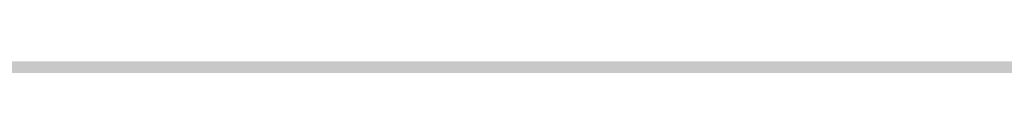
# Model space of a CAD drawing. Units: millimetres. Extents: x 0 to 2267, y 0 to 1823.
# Tile 153 of 256: x 1833.606 to 1838.83, y 1127.393 to 1127.412. Entities that reach past the tile are written whole.
import ezdxf

# ---------------------------------------------------------------- set-up
doc = ezdxf.new("R2010")
doc.units = ezdxf.units.MM
doc.header["$MEASUREMENT"] = 0
doc.layers.add('M-DIMS', color=2, linetype='Continuous', lineweight=25)
doc.layers.add('M-HATC', color=252, linetype='Continuous', lineweight=18)
doc.styles.get("Standard").update_dxf_attribs({"font": 'arial.ttf'})
doc.dimstyles.get("Standard").update_dxf_attribs({"dimtxt": 7, "dimasz": 4, "dimexe": 0.18, "dimexo": 0.0625, "dimgap": 0.09, "dimtad": 0, "dimdec": 0, "dimzin": 0, "dimdsep": 46, "dimtxsty": 'Standard', "dimcen": 0.09, "dimadec": 0, "dimazin": 0, "dimtfac": 1, "dimtdec": 0, "dimtofl": 0, "dimtmove": 0, "dimatfit": 3, "dimfxl": 1, "dimtolj": 1, "dimtzin": 0, "dimarcsym": 0})

# ---------------------------------------------------------------- blocks, each defined once
blk = doc.blocks.new('*D1')
at = {"layer": 'Defpoints', "color": 0, "transparency": 16777216}
for p in [(1593.4289, 1127.4171), (1843.4289, 1127.4171), (1843.4289, 955.6278)]:
    blk.add_point(p, dxfattribs=at)
at = {"layer": 'M-DIMS', "color": 0, "lineweight": -2, "transparency": 16777216}
for p, q in [((1593.4289, 1127.3546), (1593.4289, 955.4478)), ((1843.4289, 1127.3546), (1843.4289, 955.4478)), ((1597.4289, 955.6278), (1710.5582, 955.6278)), ((1839.4289, 955.6278), (1726.2996, 955.6278))]:
    blk.add_line(p, q, dxfattribs=at)
at = {"layer": 'M-DIMS', "color": 0, "transparency": 16777216}
for points in [[(1597.4289, 956.2944), (1597.4289, 954.9611), (1593.4289, 955.6278)], [(1839.4289, 956.2944), (1839.4289, 954.9611), (1843.4289, 955.6278)]]:
    blk.add_solid(points, dxfattribs=at)
at = {"layer": 'M-DIMS', "color": 0, "transparency": 16777216, "insert": (1718.4289, 955.6278), "char_height": 7, "attachment_point": 5}
blk.add_mtext('\\A1;250', dxfattribs=at)

msp = doc.modelspace()

# ---------------------------------------------------------------- hatches: boundary and pattern name
at = {"layer": 'M-HATC'}
h = msp.add_hatch(color=256, dxfattribs=at)
h.dxf.hatch_style = 1
h.paths.add_polyline_path([(2055.771, 1603.062), (1381.0868, 1603.062), (1381.0868, 1598.062), (2055.771, 1598.062)])
h.paths.add_polyline_path([(2055.771, 1598.062), (1381.0868, 1598.062), (1381.0868, 1593.062), (2055.771, 1593.062)])
h.paths.add_polyline_path([(2051.3074, 1536.7609), (1385.5504, 1536.7609), (1385.5504, 1526.7609), (1387.5504, 1526.7609), (1388.5366, 1525.0528), (1385.3319, 1521.2335), (1385.3319, 1521.2226), (2050.2542, 1522.7491), (2048.3212, 1525.0528), (2049.3074, 1526.7609), (2051.3074, 1526.7609)])
edge = h.paths.add_edge_path()
edge.add_arc((1847.5345, 1379.1492), 135, 222.603061, 222.890851, ccw=False)
edge.add_line((1748.1663, 1287.7656), (1683.0921, 1287.7656))
edge.add_arc((1583.7239, 1379.1492), 135, 317.109149, 317.396939, ccw=False)
edge.add_arc((1678.9686, 1290.6707), 5, 222.8909, 317.1091, ccw=False)
edge.add_arc((1774.2133, 1379.1492), 135, 222.603061, 222.890851, ccw=False)
edge.add_line((1674.8451, 1287.7656), (1609.7709, 1287.7656))
edge.add_arc((1510.4027, 1379.1492), 135, 317.109149, 317.396939, ccw=False)
edge.add_arc((1605.6474, 1290.6707), 5, 222.8909, 317.1091, ccw=False)
edge.add_arc((1700.8921, 1379.1492), 135, 222.603061, 222.890851, ccw=False)
edge.add_line((1601.5239, 1287.7656), (1536.4497, 1287.7656))
edge.add_arc((1437.0815, 1379.1492), 135, 317.109149, 317.396939, ccw=False)
edge.add_arc((1532.3262, 1290.6707), 5, 222.8909, 317.1091, ccw=False)
edge.add_arc((1627.5709, 1379.1492), 135, 222.603061, 222.890851, ccw=False)
edge.add_line((1528.2027, 1287.7656), (1505.9289, 1287.7656))
edge.add_spline(control_points=[(1505.9289, 1287.7656), (1504.2622, 1287.7656), (1504.2622, 1282.7656), (1505.9289, 1282.7656)], knot_values=[0, 0, 0, 0, 5, 5, 5, 5], degree=3, periodic=0)
edge.add_line((1505.9289, 1282.7656), (1930.9289, 1282.7656))
edge.add_spline(control_points=[(1930.9289, 1282.7656), (1932.5956, 1282.7656), (1932.5956, 1287.7656), (1930.9289, 1287.7656)], knot_values=[0, 0, 0, 0, 5, 5, 5, 5], degree=3, periodic=0)
edge.add_line((1930.9289, 1287.7656), (1903.0557, 1287.7656))
edge.add_arc((1803.6875, 1379.1492), 135, 317.109149, 317.396939, ccw=False)
edge.add_arc((1898.9322, 1290.6707), 5, 222.8909, 317.1091, ccw=False)
edge.add_arc((1994.1769, 1379.1492), 135, 222.603061, 222.890851, ccw=False)
edge.add_line((1894.8087, 1287.7656), (1829.7345, 1287.7656))
edge.add_arc((1730.3663, 1379.1492), 135, 317.109149, 317.396939, ccw=False)
edge.add_arc((1825.611, 1290.6707), 5, 222.8909, 317.1091, ccw=False)
edge.add_arc((1920.8557, 1379.1492), 135, 222.603061, 222.890851, ccw=False)
edge.add_line((1821.4875, 1287.7656), (1756.4133, 1287.7656))
edge.add_arc((1657.0451, 1379.1492), 135, 317.109149, 317.396939, ccw=False)
edge.add_arc((1752.2898, 1290.6707), 5, 222.8909, 317.1091, ccw=False)
edge = h.paths.add_edge_path()
edge.add_spline(control_points=[(1843.4289, 1227.2475), (1845.0956, 1227.2475), (1845.0956, 1232.2475), (1843.4289, 1232.2475)], knot_values=[0, 0, 0, 0, 5, 5, 5, 5], degree=3, periodic=0)
edge.add_line((1843.4289, 1232.2475), (1593.4289, 1232.2475))
edge.add_spline(control_points=[(1593.4289, 1232.2475), (1591.7622, 1232.2475), (1591.7622, 1227.2475), (1593.4289, 1227.2475)], knot_values=[0, 0, 0, 0, 5, 5, 5, 5], degree=3, periodic=0)
edge.add_line((1593.4289, 1227.2475), (1843.4289, 1227.2475))
h.paths.add_polyline_path([(1905.9289, 1127.4171), (1530.9289, 1127.4171, 0.414214), (1520.9289, 1117.4171), (1530.9289, 1117.4171), (1915.9289, 1117.4171, 0.414214)])
edge = h.paths.add_edge_path()
edge.add_arc((1397.0858, 1498.4078), 12.7299, 90.78215, 190.87871, ccw=False)
edge.add_line((1396.912, 1511.1365), (1428.0097, 1511.3488))
edge.add_line((1428.0097, 1511.3488), (1433.0097, 1511.3488))
edge.add_line((1433.0097, 1511.3488), (1434.439, 1511.3488))
edge.add_arc((1419.474, 1498.0804), 20, 41.561, 74.08211)
edge.add_line((1424.9592, 1517.3135), (1399.9351, 1517.2561))
edge.add_spline(control_points=[(1399.9307, 1517.2561), (1399.884, 1517.2131), (1399.8328, 1517.1689), (1399.7774, 1517.1236)], knot_values=[11.567499, 11.567499, 11.567499, 11.567499, 11.814249, 11.814249, 11.814249, 11.814249], degree=3, periodic=0)
edge.add_spline(control_points=[(1399.6328, 1517.0099), (1399.5831, 1516.9721), (1399.5307, 1516.9338), (1399.4759, 1516.8947)], knot_values=[11.167718, 11.167718, 11.167718, 11.167718, 11.365188, 11.365188, 11.365188, 11.365188], degree=3, periodic=0)
edge.add_spline(control_points=[(1399.3398, 1516.8001), (1399.1514, 1516.6719), (1398.9384, 1516.5377), (1398.704, 1516.3994)], knot_values=[10.376405, 10.376405, 10.376405, 10.376405, 11.00994, 11.00994, 11.00994, 11.00994], degree=3, periodic=0)
edge.add_spline(control_points=[(1398.6572, 1516.3719), (1398.5789, 1516.326), (1398.4983, 1516.2797), (1398.4155, 1516.2331)], knot_values=[10.125175, 10.125175, 10.125175, 10.125175, 10.334406, 10.334406, 10.334406, 10.334406], degree=3, periodic=0)
edge.add_spline(control_points=[(1398.2642, 1516.1487), (1398.196, 1516.1111), (1398.1263, 1516.0732), (1398.0555, 1516.0351)], knot_values=[9.832246, 9.832246, 9.832246, 9.832246, 9.999658, 9.999658, 9.999658, 9.999658], degree=3, periodic=0)
edge.add_spline(control_points=[(1397.9987, 1516.0048), (1397.7312, 1515.8621), (1397.446, 1515.7171), (1397.1466, 1515.5714)], knot_values=[9.161808, 9.161808, 9.161808, 9.161808, 9.787769, 9.787769, 9.787769, 9.787769], degree=3, periodic=0)
edge.add_spline(control_points=[(1397.1466, 1515.5714), (1396.8418, 1515.423), (1396.5222, 1515.274), (1396.1914, 1515.1262)], knot_values=[8.524455, 8.524455, 8.524455, 8.524455, 9.161808, 9.161808, 9.161808, 9.161808], degree=3, periodic=0)
edge.add_spline(control_points=[(1396.0777, 1515.0756), (1395.9854, 1515.0348), (1395.8922, 1514.994), (1395.7983, 1514.9534)], knot_values=[8.275193, 8.275193, 8.275193, 8.275193, 8.451726, 8.451726, 8.451726, 8.451726], degree=3, periodic=0)
edge.add_spline(control_points=[(1395.6018, 1514.8691), (1395.4997, 1514.8257), (1395.3968, 1514.7824), (1395.2932, 1514.7394)], knot_values=[7.962917, 7.962917, 7.962917, 7.962917, 8.152764, 8.152764, 8.152764, 8.152764], degree=3, periodic=0)
edge.add_spline(control_points=[(1395.2116, 1514.7057), (1394.8278, 1514.5475), (1394.4345, 1514.3929), (1394.0364, 1514.2442)], knot_values=[7.21254, 7.21254, 7.21254, 7.21254, 7.913148, 7.913148, 7.913148, 7.913148], degree=3, periodic=0)
edge.add_spline(control_points=[(1394.0364, 1514.2442), (1393.7076, 1514.1214), (1393.3754, 1514.0027), (1393.0427, 1513.8895)], knot_values=[6.633733, 6.633733, 6.633733, 6.633733, 7.21254, 7.21254, 7.21254, 7.21254], degree=3, periodic=0)
edge.add_spline(control_points=[(1392.8214, 1513.815), (1392.7198, 1513.7812), (1392.6181, 1513.7479), (1392.5166, 1513.7152)], knot_values=[6.328796, 6.328796, 6.328796, 6.328796, 6.505493, 6.505493, 6.505493, 6.505493], degree=3, periodic=0)
edge.add_spline(control_points=[(1392.5166, 1513.7152), (1392.3187, 1513.6515), (1392.1212, 1513.59), (1391.9244, 1513.531)], knot_values=[5.984605, 5.984605, 5.984605, 5.984605, 6.328796, 6.328796, 6.328796, 6.328796], degree=3, periodic=0)
edge.add_spline(control_points=[(1391.7915, 1513.4915), (1391.3122, 1513.3501), (1390.8384, 1513.2239), (1390.3784, 1513.1171)], knot_values=[5.066697, 5.066697, 5.066697, 5.066697, 5.907055, 5.907055, 5.907055, 5.907055], degree=3, periodic=0)
edge.add_spline(control_points=[(1390.3784, 1513.1171), (1390.1797, 1513.071), (1389.9836, 1513.0284), (1389.7907, 1512.9899)], knot_values=[4.70367, 4.70367, 4.70367, 4.70367, 5.066695, 5.066695, 5.066695, 5.066695], degree=3, periodic=0)
edge.add_spline(control_points=[(1389.422, 1512.9204), (1389.2459, 1512.8892), (1389.0729, 1512.8617), (1388.9036, 1512.8381)], knot_values=[4.130571, 4.130571, 4.130571, 4.130571, 4.469816, 4.469816, 4.469816, 4.469816], degree=3, periodic=0)
edge.add_spline(control_points=[(1388.9036, 1512.8381), (1388.591, 1512.7946), (1388.2911, 1512.7644), (1388.0071, 1512.7494)], knot_values=[3.504031, 3.504031, 3.504031, 3.504031, 4.130571, 4.130571, 4.130571, 4.130571], degree=3, periodic=0)
edge.add_spline(control_points=[(1387.9356, 1512.7459), (1387.8538, 1512.7423), (1387.7733, 1512.74), (1387.6944, 1512.739)], knot_values=[3.268866, 3.268866, 3.268866, 3.268866, 3.451164, 3.451164, 3.451164, 3.451164], degree=3, periodic=0)
edge.add_spline(control_points=[(1387.3351, 1512.7443), (1387.2076, 1512.7499), (1387.0847, 1512.7597), (1386.967, 1512.7739)], knot_values=[2.670686, 2.670686, 2.670686, 2.670686, 2.984, 2.984, 2.984, 2.984], degree=3, periodic=0)
edge.add_spline(control_points=[(1386.8327, 1512.7922), (1386.8209, 1512.7941), (1386.8092, 1512.7959), (1386.7975, 1512.7979)], knot_values=[2.516981, 2.516981, 2.516981, 2.516981, 2.549528, 2.549528, 2.549528, 2.549528], degree=3, periodic=0)
edge.add_spline(control_points=[(1386.4526, 1512.8735), (1386.4257, 1512.881), (1386.3993, 1512.889), (1386.3733, 1512.8972)], knot_values=[2.095869, 2.095869, 2.095869, 2.095869, 2.17941, 2.17941, 2.17941, 2.17941], degree=3, periodic=0)
edge.add_spline(control_points=[(1386.0691, 1513.0189), (1386.0634, 1513.0217), (1386.0577, 1513.0246), (1386.052, 1513.0275)], knot_values=[1.72453, 1.72453, 1.72453, 1.72453, 1.745933, 1.745933, 1.745933, 1.745933], degree=3, periodic=0)
edge.add_arc((1399.474, 1498.0804), 20, 131.82432, 180)
edge.add_arc((1630.3336, 1505.5484), 250.9708, 181.705176, 236.427975)
edge.add_arc((1605.3399, 1483.3044), 218.7822, 238.660829, 243.34961)
edge.add_arc((1647.0911, 1510.3592), 262.8986, 183.129836, 237.853442, ccw=False)
h.paths.add_polyline_path([(1406.5369, 1391.9644, 0.149382), (1491.5506, 1296.4418, -0.129517)], flags=17)
edge = h.paths.add_edge_path()
edge.add_arc((2037.3838, 1498.0804), 20, 0, 48.26587)
edge.add_spline(control_points=[(2050.6973, 1513.0052), (2050.6512, 1512.9847), (2050.6034, 1512.9655), (2050.5539, 1512.9477)], knot_values=[1.835652, 1.835652, 1.835652, 1.835652, 2.000781, 2.000781, 2.000781, 2.000781], degree=3, periodic=0)
edge.add_spline(control_points=[(2050.4616, 1512.9166), (2050.479, 1512.9221), (2050.4963, 1512.9277), (2050.5133, 1512.9335)], knot_values=[2.045477, 2.045477, 2.045477, 2.045477, 2.101389, 2.101389, 2.101389, 2.101389], degree=3, periodic=0)
edge.add_spline(control_points=[(2050.129, 1512.8342), (2050.1984, 1512.8473), (2050.2657, 1512.8623), (2050.3308, 1512.8792)], knot_values=[2.237629, 2.237629, 2.237629, 2.237629, 2.435841, 2.435841, 2.435841, 2.435841], degree=3, periodic=0)
edge.add_spline(control_points=[(2050.0946, 1512.8278), (2050.1061, 1512.8299), (2050.1176, 1512.832), (2050.129, 1512.8342)], knot_values=[2.435841, 2.435841, 2.435841, 2.435841, 2.468321, 2.468321, 2.468321, 2.468321], degree=3, periodic=0)
edge.add_spline(control_points=[(2049.7843, 1512.7851), (2049.8552, 1512.7922), (2049.9243, 1512.8008), (2049.9917, 1512.8109)], knot_values=[2.563852, 2.563852, 2.563852, 2.563852, 2.748541, 2.748541, 2.748541, 2.748541], degree=3, periodic=0)
edge.add_spline(control_points=[(2049.4052, 1512.7617), (2049.5364, 1512.7653), (2049.6629, 1512.773), (2049.7843, 1512.7851)], knot_values=[2.748541, 2.748541, 2.748541, 2.748541, 3.064882, 3.064882, 3.064882, 3.064882], degree=3, periodic=0)
edge.add_spline(control_points=[(2049.1698, 1512.7597), (2049.2336, 1512.7591), (2049.2965, 1512.7594), (2049.3584, 1512.7606)], knot_values=[3.102309, 3.102309, 3.102309, 3.102309, 3.2503, 3.2503, 3.2503, 3.2503], degree=3, periodic=0)
edge.add_spline(control_points=[(2048.8573, 1512.7691), (2048.9638, 1512.7638), (2049.068, 1512.7606), (2049.1698, 1512.7597)], knot_values=[3.2503, 3.2503, 3.2503, 3.2503, 3.486069, 3.486069, 3.486069, 3.486069], degree=3, periodic=0)
edge.add_spline(control_points=[(2048.6924, 1512.7789), (2048.3729, 1512.8009), (2048.0345, 1512.8411), (2047.6817, 1512.897)], knot_values=[3.606429, 3.606429, 3.606429, 3.606429, 4.2989, 4.2989, 4.2989, 4.2989], degree=3, periodic=0)
edge.add_spline(control_points=[(2047.6817, 1512.897), (2047.5458, 1512.9185), (2047.4077, 1512.9424), (2047.2678, 1512.9685)], knot_values=[4.2989, 4.2989, 4.2989, 4.2989, 4.565769, 4.565769, 4.565769, 4.565769], degree=3, periodic=0)
edge.add_spline(control_points=[(2047.2678, 1512.9685), (2047.1449, 1512.9914), (2047.0207, 1513.016), (2046.8951, 1513.0422)], knot_values=[4.565769, 4.565769, 4.565769, 4.565769, 4.799971, 4.799971, 4.799971, 4.799971], degree=3, periodic=0)
edge.add_spline(control_points=[(2046.8951, 1513.0422), (2046.5286, 1513.1188), (2046.1513, 1513.209), (2045.7676, 1513.3107)], knot_values=[4.799971, 4.799971, 4.799971, 4.799971, 5.483718, 5.483718, 5.483718, 5.483718], degree=3, periodic=0)
edge.add_spline(control_points=[(2045.7676, 1513.3107), (2045.3724, 1513.4154), (2044.9704, 1513.5322), (2044.5662, 1513.6588)], knot_values=[5.483718, 5.483718, 5.483718, 5.483718, 6.187866, 6.187866, 6.187866, 6.187866], degree=3, periodic=0)
edge.add_spline(control_points=[(2044.5662, 1513.6588), (2044.4149, 1513.7061), (2044.2633, 1513.7549), (2044.1116, 1513.8048)], knot_values=[6.187866, 6.187866, 6.187866, 6.187866, 6.451551, 6.451551, 6.451551, 6.451551], degree=3, periodic=0)
edge.add_spline(control_points=[(2044.1116, 1513.8048), (2043.9967, 1513.8427), (2043.8817, 1513.8813), (2043.7668, 1513.9205)], knot_values=[6.451551, 6.451551, 6.451551, 6.451551, 6.651434, 6.651434, 6.651434, 6.651434], degree=3, periodic=0)
edge.add_spline(control_points=[(2043.7668, 1513.9205), (2043.3716, 1514.0554), (2042.9774, 1514.1979), (2042.5886, 1514.3458)], knot_values=[6.651434, 6.651434, 6.651434, 6.651434, 7.338879, 7.338879, 7.338879, 7.338879], degree=3, periodic=0)
edge.add_spline(control_points=[(2042.5886, 1514.3458), (2042.1643, 1514.5071), (2041.7465, 1514.6749), (2041.3409, 1514.846)], knot_values=[7.338879, 7.338879, 7.338879, 7.338879, 8.089209, 8.089209, 8.089209, 8.089209], degree=3, periodic=0)
edge.add_spline(control_points=[(2041.3409, 1514.846), (2041.1028, 1514.9465), (2040.869, 1515.0481), (2040.6405, 1515.1502)], knot_values=[8.089209, 8.089209, 8.089209, 8.089209, 8.529587, 8.529587, 8.529587, 8.529587], degree=3, periodic=0)
edge.add_spline(control_points=[(2040.51, 1515.2089), (2040.0824, 1515.4022), (2039.6747, 1515.5971), (2039.295, 1515.7894)], knot_values=[8.613818, 8.613818, 8.613818, 8.613818, 9.44571, 9.44571, 9.44571, 9.44571], degree=3, periodic=0)
edge.add_spline(control_points=[(2039.295, 1515.7894), (2039.0618, 1515.9075), (2038.8391, 1516.0246), (2038.6288, 1516.1398)], knot_values=[9.44571, 9.44571, 9.44571, 9.44571, 9.956404, 9.956404, 9.956404, 9.956404], degree=3, periodic=0)
edge.add_spline(control_points=[(2038.6288, 1516.1398), (2038.5187, 1516.2001), (2038.4121, 1516.2598), (2038.309, 1516.3189)], knot_values=[9.956404, 9.956404, 9.956404, 9.956404, 10.223542, 10.223542, 10.223542, 10.223542], degree=3, periodic=0)
edge.add_spline(control_points=[(2038.309, 1516.3189), (2038.2138, 1516.3735), (2038.1216, 1516.4276), (2038.0328, 1516.481)], knot_values=[10.223542, 10.223542, 10.223542, 10.223542, 10.47051, 10.47051, 10.47051, 10.47051], degree=3, periodic=0)
edge.add_spline(control_points=[(2038.0328, 1516.481), (2037.7855, 1516.6296), (2037.5639, 1516.773), (2037.3722, 1516.909)], knot_values=[10.47051, 10.47051, 10.47051, 10.47051, 11.15767, 11.15767, 11.15767, 11.15767], degree=3, periodic=0)
edge.add_spline(control_points=[(2037.3722, 1516.909), (2037.2789, 1516.9752), (2037.1927, 1517.0396), (2037.1142, 1517.102)], knot_values=[11.15767, 11.15767, 11.15767, 11.15767, 11.49227, 11.49227, 11.49227, 11.49227], degree=3, periodic=0)
edge.add_spline(control_points=[(2036.8564, 1517.3259), (2036.9148, 1517.2692), (2036.9814, 1517.2103), (2037.0557, 1517.1492)], knot_values=[11.577341, 11.577341, 11.577341, 11.577341, 11.91035, 11.91035, 11.91035, 11.91035], degree=3, periodic=0)
edge.add_spline(control_points=[(2036.8074, 1517.3748), (2036.823, 1517.3587), (2036.8393, 1517.3424), (2036.8564, 1517.3259)], knot_values=[11.91035, 11.91035, 11.91035, 11.91035, 12.007402, 12.007402, 12.007402, 12.007402], degree=3, periodic=0)
edge.add_spline(control_points=[(2036.7017, 1517.494), (2036.7104, 1517.483), (2036.7196, 1517.4719), (2036.7291, 1517.4606)], knot_values=[12.184155, 12.184155, 12.184155, 12.184155, 12.255409, 12.255409, 12.255409, 12.255409], degree=3, periodic=0)
edge.add_spline(control_points=[(2036.6159, 1517.6205), (2036.62, 1517.613), (2036.6243, 1517.6055), (2036.6289, 1517.5979)], knot_values=[12.487913, 12.487913, 12.487913, 12.487913, 12.541035, 12.541035, 12.541035, 12.541035], degree=3, periodic=0)
edge.add_spline(control_points=[(2036.5635, 1517.786), (2036.5637, 1517.7794), (2036.5642, 1517.7726), (2036.565, 1517.7658)], knot_values=[12.911761, 12.911761, 12.911761, 12.911761, 12.968286, 12.968286, 12.968286, 12.968286], degree=3, periodic=0)
edge.add_spline(control_points=[(2036.6166, 1517.9304), (2036.6125, 1517.9259), (2036.6086, 1517.9212), (2036.6049, 1517.9165)], knot_values=[13.382527, 13.382527, 13.382527, 13.382527, 13.433791, 13.433791, 13.433791, 13.433791], degree=3, periodic=0)
edge.add_spline(control_points=[(2036.749, 1518.017), (2036.7361, 1518.0116), (2036.7239, 1518.006), (2036.7124, 1518.0002)], knot_values=[13.726299, 13.726299, 13.726299, 13.726299, 13.809928, 13.809928, 13.809928, 13.809928], degree=3, periodic=0)
edge.add_spline(control_points=[(2036.8604, 1518.0528), (2036.8386, 1518.0474), (2036.8181, 1518.0416), (2036.7988, 1518.0353)], knot_values=[13.910887, 13.910887, 13.910887, 13.910887, 14.02153, 14.02153, 14.02153, 14.02153], degree=3, periodic=0)
edge.add_line((2036.9639, 1518.0804), (2032.3838, 1518.0804))
edge.add_line((2032.3838, 1518.0804), (2027.3838, 1518.0804))
edge.add_line((2027.3838, 1518.0804), (2022.3838, 1518.0804))
edge.add_line((2022.3838, 1518.0804), (2017.3838, 1518.0804))
edge.add_arc((2017.3838, 1498.0804), 20, 90, 138.439)
edge.add_line((2002.4188, 1511.3488), (2003.8481, 1511.3488))
edge.add_line((2003.8481, 1511.3488), (2008.8481, 1511.3488))
edge.add_line((2008.8481, 1511.3488), (2039.772, 1511.1377))
edge.add_arc((2039.772, 1498.4078), 12.7299, -10.87871, 90, ccw=False)
edge.add_arc((1789.7668, 1510.3592), 262.8986, 302.146558, 356.870164, ccw=False)
edge.add_arc((1831.5179, 1483.3044), 218.7822, 296.65039, 301.339171)
edge.add_arc((1806.5242, 1505.5484), 250.9708, 303.572025, 358.294824)
h.paths.add_polyline_path([(2030.321, 1391.9644, -0.129517), (1945.3072, 1296.4418, 0.149382)], flags=17)
edge = h.paths.add_edge_path()
edge.add_spline(control_points=[(2037.2464, 1518.0821), (2037.2898, 1518.081), (2037.3355, 1518.0804), (2037.3838, 1518.0804)], knot_values=[0.000012, 0.000012, 0.000012, 0.000012, 0.144754, 0.144754, 0.144754, 0.144754], degree=3, periodic=0)
edge.add_line((2037.3357, 1518.0804), (2037.0096, 1518.0804))
edge.add_spline(control_points=[(2037.0096, 1518.0804), (2036.9822, 1518.0768), (2036.956, 1518.0727), (2036.9312, 1518.0681)], knot_values=[14.13465, 14.13465, 14.13465, 14.13465, 14.247197, 14.247197, 14.247197, 14.247197], degree=3, periodic=0)
edge.add_spline(control_points=[(2036.9312, 1518.0681), (2036.9276, 1518.0674), (2036.9241, 1518.0667), (2036.9205, 1518.0661)], knot_values=[14.118315, 14.118315, 14.118315, 14.118315, 14.13465, 14.13465, 14.13465, 14.13465], degree=3, periodic=0)
edge.add_spline(control_points=[(2036.9205, 1518.0661), (2036.9118, 1518.0644), (2036.9032, 1518.0626), (2036.8948, 1518.0608)], knot_values=[14.078086, 14.078086, 14.078086, 14.078086, 14.118315, 14.118315, 14.118315, 14.118315], degree=3, periodic=0)
edge.add_spline(control_points=[(2036.8948, 1518.0608), (2036.883, 1518.0583), (2036.8716, 1518.0556), (2036.8604, 1518.0528)], knot_values=[14.02153, 14.02153, 14.02153, 14.02153, 14.078086, 14.078086, 14.078086, 14.078086], degree=3, periodic=0)
edge.add_spline(control_points=[(2036.8604, 1518.0528), (2036.8386, 1518.0474), (2036.8181, 1518.0416), (2036.7988, 1518.0353)], knot_values=[13.910887, 13.910887, 13.910887, 13.910887, 14.02153, 14.02153, 14.02153, 14.02153], degree=3, periodic=0)
edge.add_spline(control_points=[(2036.7988, 1518.0353), (2036.7981, 1518.035), (2036.7974, 1518.0348), (2036.7967, 1518.0346)], knot_values=[13.906906, 13.906906, 13.906906, 13.906906, 13.910887, 13.910887, 13.910887, 13.910887], degree=3, periodic=0)
edge.add_spline(control_points=[(2036.7967, 1518.0346), (2036.7882, 1518.0318), (2036.7799, 1518.0289), (2036.7719, 1518.0259)], knot_values=[13.857826, 13.857826, 13.857826, 13.857826, 13.906906, 13.906906, 13.906906, 13.906906], degree=3, periodic=0)
edge.add_spline(control_points=[(2036.7719, 1518.0259), (2036.764, 1518.023), (2036.7564, 1518.02), (2036.749, 1518.017)], knot_values=[13.809928, 13.809928, 13.809928, 13.809928, 13.857826, 13.857826, 13.857826, 13.857826], degree=3, periodic=0)
edge.add_spline(control_points=[(2036.749, 1518.017), (2036.7361, 1518.0116), (2036.7239, 1518.006), (2036.7124, 1518.0002)], knot_values=[13.726299, 13.726299, 13.726299, 13.726299, 13.809928, 13.809928, 13.809928, 13.809928], degree=3, periodic=0)
edge.add_spline(control_points=[(2036.7124, 1518.0002), (2036.7121, 1518), (2036.7118, 1517.9999), (2036.7115, 1517.9997)], knot_values=[13.723993, 13.723993, 13.723993, 13.723993, 13.726299, 13.726299, 13.726299, 13.726299], degree=3, periodic=0)
edge.add_spline(control_points=[(2036.7115, 1517.9997), (2036.7063, 1517.9971), (2036.7013, 1517.9944), (2036.6965, 1517.9917)], knot_values=[13.686536, 13.686536, 13.686536, 13.686536, 13.723993, 13.723993, 13.723993, 13.723993], degree=3, periodic=0)
edge.add_spline(control_points=[(2036.6965, 1517.9917), (2036.6919, 1517.9891), (2036.6874, 1517.9865), (2036.6831, 1517.9839)], knot_values=[13.651251, 13.651251, 13.651251, 13.651251, 13.686536, 13.686536, 13.686536, 13.686536], degree=3, periodic=0)
edge.add_spline(control_points=[(2036.6831, 1517.9839), (2036.6764, 1517.9798), (2036.67, 1517.9757), (2036.6639, 1517.9714)], knot_values=[13.596804, 13.596804, 13.596804, 13.596804, 13.651251, 13.651251, 13.651251, 13.651251], degree=3, periodic=0)
edge.add_spline(control_points=[(2036.6639, 1517.9714), (2036.6636, 1517.9712), (2036.6633, 1517.9709), (2036.6629, 1517.9707)], knot_values=[13.593956, 13.593956, 13.593956, 13.593956, 13.596804, 13.596804, 13.596804, 13.596804], degree=3, periodic=0)
edge.add_spline(control_points=[(2036.6629, 1517.9707), (2036.6603, 1517.9689), (2036.6577, 1517.967), (2036.6552, 1517.9651)], knot_values=[13.570322, 13.570322, 13.570322, 13.570322, 13.593956, 13.593956, 13.593956, 13.593956], degree=3, periodic=0)
edge.add_spline(control_points=[(2036.6552, 1517.9651), (2036.6525, 1517.9631), (2036.6499, 1517.9611), (2036.6474, 1517.9591)], knot_values=[13.545477, 13.545477, 13.545477, 13.545477, 13.570322, 13.570322, 13.570322, 13.570322], degree=3, periodic=0)
edge.add_spline(control_points=[(2036.6474, 1517.9591), (2036.6472, 1517.9589), (2036.6471, 1517.9588), (2036.6469, 1517.9587)], knot_values=[13.543931, 13.543931, 13.543931, 13.543931, 13.545477, 13.545477, 13.545477, 13.545477], degree=3, periodic=0)
edge.add_spline(control_points=[(2036.6469, 1517.9587), (2036.6412, 1517.9541), (2036.6358, 1517.9494), (2036.6307, 1517.9447)], knot_values=[13.488237, 13.488237, 13.488237, 13.488237, 13.543931, 13.543931, 13.543931, 13.543931], degree=3, periodic=0)
edge.add_spline(control_points=[(2036.6307, 1517.9447), (2036.6282, 1517.9423), (2036.6257, 1517.9399), (2036.6233, 1517.9374)], knot_values=[13.460307, 13.460307, 13.460307, 13.460307, 13.488237, 13.488237, 13.488237, 13.488237], degree=3, periodic=0)
edge.add_spline(control_points=[(2036.6233, 1517.9374), (2036.6215, 1517.9356), (2036.6198, 1517.9338), (2036.6181, 1517.932)], knot_values=[13.439712, 13.439712, 13.439712, 13.439712, 13.460307, 13.460307, 13.460307, 13.460307], degree=3, periodic=0)
edge.add_spline(control_points=[(2036.6181, 1517.932), (2036.6176, 1517.9315), (2036.6171, 1517.9309), (2036.6166, 1517.9304)], knot_values=[13.433791, 13.433791, 13.433791, 13.433791, 13.439712, 13.439712, 13.439712, 13.439712], degree=3, periodic=0)
edge.add_spline(control_points=[(2036.6166, 1517.9304), (2036.6125, 1517.9259), (2036.6086, 1517.9212), (2036.6049, 1517.9165)], knot_values=[13.382527, 13.382527, 13.382527, 13.382527, 13.433791, 13.433791, 13.433791, 13.433791], degree=3, periodic=0)
edge.add_spline(control_points=[(2036.6049, 1517.9165), (2036.6026, 1517.9135), (2036.6004, 1517.9104), (2036.5982, 1517.9074)], knot_values=[13.350017, 13.350017, 13.350017, 13.350017, 13.382527, 13.382527, 13.382527, 13.382527], degree=3, periodic=0)
edge.add_spline(control_points=[(2036.5982, 1517.9074), (2036.5972, 1517.9059), (2036.5962, 1517.9043), (2036.5952, 1517.9028)], knot_values=[13.333922, 13.333922, 13.333922, 13.333922, 13.350017, 13.350017, 13.350017, 13.350017], degree=3, periodic=0)
edge.add_spline(control_points=[(2036.5952, 1517.9028), (2036.5945, 1517.9018), (2036.5939, 1517.9009), (2036.5933, 1517.8999)], knot_values=[13.323828, 13.323828, 13.323828, 13.323828, 13.333922, 13.333922, 13.333922, 13.333922], degree=3, periodic=0)
edge.add_spline(control_points=[(2036.5933, 1517.8999), (2036.5905, 1517.8955), (2036.5879, 1517.8909), (2036.5855, 1517.8864)], knot_values=[13.277545, 13.277545, 13.277545, 13.277545, 13.323828, 13.323828, 13.323828, 13.323828], degree=3, periodic=0)
edge.add_spline(control_points=[(2036.5855, 1517.8864), (2036.5836, 1517.8827), (2036.5817, 1517.8789), (2036.5801, 1517.8751)], knot_values=[13.240119, 13.240119, 13.240119, 13.240119, 13.277545, 13.277545, 13.277545, 13.277545], degree=3, periodic=0)
edge.add_spline(control_points=[(2036.5801, 1517.8751), (2036.5795, 1517.8739), (2036.579, 1517.8727), (2036.5785, 1517.8715)], knot_values=[13.228211, 13.228211, 13.228211, 13.228211, 13.240119, 13.240119, 13.240119, 13.240119], degree=3, periodic=0)
edge.add_spline(control_points=[(2036.5785, 1517.8715), (2036.578, 1517.8702), (2036.5774, 1517.869), (2036.5769, 1517.8677)], knot_values=[13.215717, 13.215717, 13.215717, 13.215717, 13.228211, 13.228211, 13.228211, 13.228211], degree=3, periodic=0)
edge.add_spline(control_points=[(2036.5769, 1517.8677), (2036.5755, 1517.864), (2036.5741, 1517.8603), (2036.5729, 1517.8565)], knot_values=[13.179847, 13.179847, 13.179847, 13.179847, 13.215717, 13.215717, 13.215717, 13.215717], degree=3, periodic=0)
edge.add_spline(control_points=[(2036.5729, 1517.8565), (2036.5713, 1517.8515), (2036.5699, 1517.8464), (2036.5687, 1517.8413)], knot_values=[13.132017, 13.132017, 13.132017, 13.132017, 13.179847, 13.179847, 13.179847, 13.179847], degree=3, periodic=0)
edge.add_spline(control_points=[(2036.5687, 1517.8413), (2036.5684, 1517.8402), (2036.5682, 1517.8392), (2036.568, 1517.8382)], knot_values=[13.122482, 13.122482, 13.122482, 13.122482, 13.132017, 13.132017, 13.132017, 13.132017], degree=3, periodic=0)
edge.add_spline(control_points=[(2036.568, 1517.8382), (2036.5676, 1517.8363), (2036.5672, 1517.8345), (2036.5669, 1517.8327)], knot_values=[13.105592, 13.105592, 13.105592, 13.105592, 13.122482, 13.122482, 13.122482, 13.122482], degree=3, periodic=0)
edge.add_spline(control_points=[(2036.5669, 1517.8327), (2036.5662, 1517.8292), (2036.5657, 1517.8257), (2036.5652, 1517.8222)], knot_values=[13.074063, 13.074063, 13.074063, 13.074063, 13.105592, 13.105592, 13.105592, 13.105592], degree=3, periodic=0)
edge.add_spline(control_points=[(2036.5652, 1517.8222), (2036.5652, 1517.8222), (2036.5652, 1517.8222), (2036.5652, 1517.8222)], knot_values=[13.074043, 13.074043, 13.074043, 13.074043, 13.074063, 13.074063, 13.074063, 13.074063], degree=3, periodic=0)
edge.add_spline(control_points=[(2036.5652, 1517.8222), (2036.5644, 1517.8164), (2036.5639, 1517.8106), (2036.5636, 1517.8046)], knot_values=[13.021884, 13.021884, 13.021884, 13.021884, 13.074043, 13.074043, 13.074043, 13.074043], degree=3, periodic=0)
edge.add_spline(control_points=[(2036.5636, 1517.8046), (2036.5636, 1517.804), (2036.5636, 1517.8034), (2036.5635, 1517.8028)], knot_values=[13.01674, 13.01674, 13.01674, 13.01674, 13.021884, 13.021884, 13.021884, 13.021884], degree=3, periodic=0)
edge.add_spline(control_points=[(2036.5635, 1517.8028), (2036.5634, 1517.8005), (2036.5634, 1517.7982), (2036.5634, 1517.7958)], knot_values=[12.996438, 12.996438, 12.996438, 12.996438, 13.01674, 13.01674, 13.01674, 13.01674], degree=3, periodic=0)
edge.add_spline(control_points=[(2036.5634, 1517.7958), (2036.5633, 1517.7926), (2036.5634, 1517.7893), (2036.5635, 1517.786)], knot_values=[12.968286, 12.968286, 12.968286, 12.968286, 12.996438, 12.996438, 12.996438, 12.996438], degree=3, periodic=0)
edge.add_spline(control_points=[(2036.5635, 1517.786), (2036.5637, 1517.7794), (2036.5642, 1517.7726), (2036.565, 1517.7658)], knot_values=[12.911761, 12.911761, 12.911761, 12.911761, 12.968286, 12.968286, 12.968286, 12.968286], degree=3, periodic=0)
edge.add_spline(control_points=[(2036.565, 1517.7658), (2036.565, 1517.7657), (2036.565, 1517.7656), (2036.565, 1517.7656)], knot_values=[12.911017, 12.911017, 12.911017, 12.911017, 12.911761, 12.911761, 12.911761, 12.911761], degree=3, periodic=0)
edge.add_spline(control_points=[(2036.565, 1517.7656), (2036.5654, 1517.7625), (2036.5658, 1517.7593), (2036.5663, 1517.7562)], knot_values=[12.88528, 12.88528, 12.88528, 12.88528, 12.911017, 12.911017, 12.911017, 12.911017], degree=3, periodic=0)
edge.add_spline(control_points=[(2036.5663, 1517.7562), (2036.5667, 1517.7534), (2036.5672, 1517.7506), (2036.5677, 1517.7478)], knot_values=[12.862519, 12.862519, 12.862519, 12.862519, 12.88528, 12.88528, 12.88528, 12.88528], degree=3, periodic=0)
edge.add_spline(control_points=[(2036.5677, 1517.7478), (2036.5678, 1517.7474), (2036.5679, 1517.7469), (2036.568, 1517.7465)], knot_values=[12.858885, 12.858885, 12.858885, 12.858885, 12.862519, 12.862519, 12.862519, 12.862519], degree=3, periodic=0)
edge.add_spline(control_points=[(2036.568, 1517.7465), (2036.5692, 1517.7399), (2036.5707, 1517.7332), (2036.5724, 1517.7264)], knot_values=[12.8053, 12.8053, 12.8053, 12.8053, 12.858885, 12.858885, 12.858885, 12.858885], degree=3, periodic=0)
edge.add_spline(control_points=[(2036.5724, 1517.7264), (2036.5734, 1517.7226), (2036.5745, 1517.7187), (2036.5756, 1517.7149)], knot_values=[12.775176, 12.775176, 12.775176, 12.775176, 12.8053, 12.8053, 12.8053, 12.8053], degree=3, periodic=0)
edge.add_spline(control_points=[(2036.5756, 1517.7149), (2036.5763, 1517.7125), (2036.577, 1517.7102), (2036.5778, 1517.7078)], knot_values=[12.756759, 12.756759, 12.756759, 12.756759, 12.775176, 12.775176, 12.775176, 12.775176], degree=3, periodic=0)
edge.add_spline(control_points=[(2036.5778, 1517.7078), (2036.5781, 1517.7067), (2036.5784, 1517.7057), (2036.5787, 1517.7047)], knot_values=[12.748742, 12.748742, 12.748742, 12.748742, 12.756759, 12.756759, 12.756759, 12.756759], degree=3, periodic=0)
edge.add_spline(control_points=[(2036.5787, 1517.7047), (2036.5808, 1517.6983), (2036.5831, 1517.6919), (2036.5856, 1517.6854)], knot_values=[12.69959, 12.69959, 12.69959, 12.69959, 12.748742, 12.748742, 12.748742, 12.748742], degree=3, periodic=0)
edge.add_spline(control_points=[(2036.5856, 1517.6854), (2036.5876, 1517.68), (2036.5898, 1517.6746), (2036.5921, 1517.6692)], knot_values=[12.659038, 12.659038, 12.659038, 12.659038, 12.69959, 12.69959, 12.69959, 12.69959], degree=3, periodic=0)
edge.add_spline(control_points=[(2036.5921, 1517.6692), (2036.594, 1517.6648), (2036.5959, 1517.6605), (2036.5979, 1517.6561)], knot_values=[12.626806, 12.626806, 12.626806, 12.626806, 12.659038, 12.659038, 12.659038, 12.659038], degree=3, periodic=0)
edge.add_spline(control_points=[(2036.5979, 1517.6561), (2036.5984, 1517.6551), (2036.5989, 1517.6541), (2036.5993, 1517.6531)], knot_values=[12.619394, 12.619394, 12.619394, 12.619394, 12.626806, 12.626806, 12.626806, 12.626806], degree=3, periodic=0)
edge.add_spline(control_points=[(2036.5993, 1517.6531), (2036.6043, 1517.6424), (2036.6099, 1517.6315), (2036.6159, 1517.6205)], knot_values=[12.541039, 12.541039, 12.541039, 12.541039, 12.619394, 12.619394, 12.619394, 12.619394], degree=3, periodic=0)
edge.add_spline(control_points=[(2036.6159, 1517.6205), (2036.6159, 1517.6205), (2036.6159, 1517.6205), (2036.6159, 1517.6205)], knot_values=[12.541035, 12.541035, 12.541035, 12.541035, 12.541039, 12.541039, 12.541039, 12.541039], degree=3, periodic=0)
edge.add_spline(control_points=[(2036.6159, 1517.6205), (2036.62, 1517.613), (2036.6243, 1517.6055), (2036.6289, 1517.5979)], knot_values=[12.487913, 12.487913, 12.487913, 12.487913, 12.541035, 12.541035, 12.541035, 12.541035], degree=3, periodic=0)
edge.add_spline(control_points=[(2036.6289, 1517.5979), (2036.6326, 1517.5916), (2036.6365, 1517.5853), (2036.6406, 1517.5789)], knot_values=[12.443982, 12.443982, 12.443982, 12.443982, 12.487913, 12.487913, 12.487913, 12.487913], degree=3, periodic=0)
edge.add_spline(control_points=[(2036.6406, 1517.5789), (2036.6414, 1517.5776), (2036.6423, 1517.5763), (2036.6431, 1517.5749)], knot_values=[12.434996, 12.434996, 12.434996, 12.434996, 12.443982, 12.443982, 12.443982, 12.443982], degree=3, periodic=0)
edge.add_spline(control_points=[(2036.6431, 1517.5749), (2036.6531, 1517.5596), (2036.6639, 1517.5439), (2036.6756, 1517.528)], knot_values=[12.329647, 12.329647, 12.329647, 12.329647, 12.434996, 12.434996, 12.434996, 12.434996], degree=3, periodic=0)
edge.add_spline(control_points=[(2036.6756, 1517.528), (2036.6839, 1517.5168), (2036.6925, 1517.5055), (2036.7017, 1517.494)], knot_values=[12.255409, 12.255409, 12.255409, 12.255409, 12.329647, 12.329647, 12.329647, 12.329647], degree=3, periodic=0)
edge.add_spline(control_points=[(2036.7017, 1517.494), (2036.7104, 1517.483), (2036.7196, 1517.4719), (2036.7291, 1517.4606)], knot_values=[12.184155, 12.184155, 12.184155, 12.184155, 12.255409, 12.255409, 12.255409, 12.255409], degree=3, periodic=0)
edge.add_spline(control_points=[(2036.7291, 1517.4606), (2036.7436, 1517.4435), (2036.759, 1517.4262), (2036.7753, 1517.4085)], knot_values=[12.075961, 12.075961, 12.075961, 12.075961, 12.184155, 12.184155, 12.184155, 12.184155], degree=3, periodic=0)
edge.add_spline(control_points=[(2036.7753, 1517.4085), (2036.7763, 1517.4075), (2036.7773, 1517.4064), (2036.7783, 1517.4054)], knot_values=[12.069502, 12.069502, 12.069502, 12.069502, 12.075961, 12.075961, 12.075961, 12.075961], degree=3, periodic=0)
edge.add_spline(control_points=[(2036.7783, 1517.4054), (2036.7877, 1517.3953), (2036.7974, 1517.385), (2036.8074, 1517.3748)], knot_values=[12.007402, 12.007402, 12.007402, 12.007402, 12.069502, 12.069502, 12.069502, 12.069502], degree=3, periodic=0)
edge.add_spline(control_points=[(2036.8074, 1517.3748), (2036.823, 1517.3587), (2036.8393, 1517.3424), (2036.8564, 1517.3259)], knot_values=[11.91035, 11.91035, 11.91035, 11.91035, 12.007402, 12.007402, 12.007402, 12.007402], degree=3, periodic=0)
edge.add_spline(control_points=[(2036.8564, 1517.3259), (2036.9148, 1517.2692), (2036.9814, 1517.2103), (2037.0557, 1517.1492)], knot_values=[11.577341, 11.577341, 11.577341, 11.577341, 11.91035, 11.91035, 11.91035, 11.91035], degree=3, periodic=0)
edge.add_spline(control_points=[(2037.0557, 1517.1492), (2037.0747, 1517.1336), (2037.0942, 1517.1179), (2037.1142, 1517.102)], knot_values=[11.49227, 11.49227, 11.49227, 11.49227, 11.577341, 11.577341, 11.577341, 11.577341], degree=3, periodic=0)
edge.add_spline(control_points=[(2037.1142, 1517.102), (2037.1927, 1517.0396), (2037.2789, 1516.9752), (2037.3722, 1516.909)], knot_values=[11.15767, 11.15767, 11.15767, 11.15767, 11.49227, 11.49227, 11.49227, 11.49227], degree=3, periodic=0)
edge.add_spline(control_points=[(2037.3722, 1516.909), (2037.5639, 1516.773), (2037.7855, 1516.6296), (2038.0328, 1516.481)], knot_values=[10.47051, 10.47051, 10.47051, 10.47051, 11.15767, 11.15767, 11.15767, 11.15767], degree=3, periodic=0)
edge.add_spline(control_points=[(2038.0328, 1516.481), (2038.1216, 1516.4276), (2038.2138, 1516.3735), (2038.309, 1516.3189)], knot_values=[10.223542, 10.223542, 10.223542, 10.223542, 10.47051, 10.47051, 10.47051, 10.47051], degree=3, periodic=0)
edge.add_spline(control_points=[(2038.309, 1516.3189), (2038.4121, 1516.2598), (2038.5187, 1516.2001), (2038.6288, 1516.1398)], knot_values=[9.956404, 9.956404, 9.956404, 9.956404, 10.223542, 10.223542, 10.223542, 10.223542], degree=3, periodic=0)
edge.add_spline(control_points=[(2038.6288, 1516.1398), (2038.8391, 1516.0246), (2039.0618, 1515.9075), (2039.295, 1515.7894)], knot_values=[9.44571, 9.44571, 9.44571, 9.44571, 9.956404, 9.956404, 9.956404, 9.956404], degree=3, periodic=0)
edge.add_spline(control_points=[(2039.295, 1515.7894), (2039.6747, 1515.5971), (2040.0824, 1515.4022), (2040.51, 1515.2089)], knot_values=[8.613818, 8.613818, 8.613818, 8.613818, 9.44571, 9.44571, 9.44571, 9.44571], degree=3, periodic=0)
edge.add_spline(control_points=[(2040.51, 1515.2089), (2040.5533, 1515.1893), (2040.5968, 1515.1697), (2040.6405, 1515.1502)], knot_values=[8.529587, 8.529587, 8.529587, 8.529587, 8.613818, 8.613818, 8.613818, 8.613818], degree=3, periodic=0)
edge.add_spline(control_points=[(2040.6405, 1515.1502), (2040.869, 1515.0481), (2041.1028, 1514.9465), (2041.3409, 1514.846)], knot_values=[8.089209, 8.089209, 8.089209, 8.089209, 8.529587, 8.529587, 8.529587, 8.529587], degree=3, periodic=0)
edge.add_spline(control_points=[(2041.3409, 1514.846), (2041.7465, 1514.6749), (2042.1643, 1514.5071), (2042.5886, 1514.3458)], knot_values=[7.338879, 7.338879, 7.338879, 7.338879, 8.089209, 8.089209, 8.089209, 8.089209], degree=3, periodic=0)
edge.add_spline(control_points=[(2042.5886, 1514.3458), (2042.9774, 1514.1979), (2043.3716, 1514.0554), (2043.7668, 1513.9205)], knot_values=[6.651434, 6.651434, 6.651434, 6.651434, 7.338879, 7.338879, 7.338879, 7.338879], degree=3, periodic=0)
edge.add_spline(control_points=[(2043.7668, 1513.9205), (2043.8817, 1513.8813), (2043.9967, 1513.8427), (2044.1116, 1513.8048)], knot_values=[6.451551, 6.451551, 6.451551, 6.451551, 6.651434, 6.651434, 6.651434, 6.651434], degree=3, periodic=0)
edge.add_spline(control_points=[(2044.1116, 1513.8048), (2044.2633, 1513.7549), (2044.4149, 1513.7061), (2044.5662, 1513.6588)], knot_values=[6.187866, 6.187866, 6.187866, 6.187866, 6.451551, 6.451551, 6.451551, 6.451551], degree=3, periodic=0)
edge.add_spline(control_points=[(2044.5662, 1513.6588), (2044.9704, 1513.5322), (2045.3724, 1513.4154), (2045.7676, 1513.3107)], knot_values=[5.483718, 5.483718, 5.483718, 5.483718, 6.187866, 6.187866, 6.187866, 6.187866], degree=3, periodic=0)
edge.add_spline(control_points=[(2045.7676, 1513.3107), (2046.1513, 1513.209), (2046.5286, 1513.1188), (2046.8951, 1513.0422)], knot_values=[4.799971, 4.799971, 4.799971, 4.799971, 5.483718, 5.483718, 5.483718, 5.483718], degree=3, periodic=0)
edge.add_spline(control_points=[(2046.8951, 1513.0422), (2047.0207, 1513.016), (2047.1449, 1512.9914), (2047.2678, 1512.9685)], knot_values=[4.565769, 4.565769, 4.565769, 4.565769, 4.799971, 4.799971, 4.799971, 4.799971], degree=3, periodic=0)
edge.add_spline(control_points=[(2047.2678, 1512.9685), (2047.4077, 1512.9424), (2047.5458, 1512.9185), (2047.6817, 1512.897)], knot_values=[4.2989, 4.2989, 4.2989, 4.2989, 4.565769, 4.565769, 4.565769, 4.565769], degree=3, periodic=0)
edge.add_spline(control_points=[(2047.6817, 1512.897), (2048.0345, 1512.8411), (2048.3729, 1512.8009), (2048.6924, 1512.7789)], knot_values=[3.606429, 3.606429, 3.606429, 3.606429, 4.2989, 4.2989, 4.2989, 4.2989], degree=3, periodic=0)
edge.add_spline(control_points=[(2048.6924, 1512.7789), (2048.7479, 1512.7751), (2048.8029, 1512.7718), (2048.8573, 1512.7691)], knot_values=[3.486069, 3.486069, 3.486069, 3.486069, 3.606429, 3.606429, 3.606429, 3.606429], degree=3, periodic=0)
edge.add_spline(control_points=[(2048.8573, 1512.7691), (2048.9638, 1512.7638), (2049.068, 1512.7606), (2049.1698, 1512.7597)], knot_values=[3.2503, 3.2503, 3.2503, 3.2503, 3.486069, 3.486069, 3.486069, 3.486069], degree=3, periodic=0)
edge.add_spline(control_points=[(2049.1698, 1512.7597), (2049.2336, 1512.7591), (2049.2965, 1512.7594), (2049.3584, 1512.7606)], knot_values=[3.102309, 3.102309, 3.102309, 3.102309, 3.2503, 3.2503, 3.2503, 3.2503], degree=3, periodic=0)
edge.add_spline(control_points=[(2049.3584, 1512.7606), (2049.3741, 1512.7609), (2049.3897, 1512.7613), (2049.4052, 1512.7617)], knot_values=[3.064882, 3.064882, 3.064882, 3.064882, 3.102309, 3.102309, 3.102309, 3.102309], degree=3, periodic=0)
edge.add_spline(control_points=[(2049.4052, 1512.7617), (2049.5364, 1512.7653), (2049.6629, 1512.773), (2049.7843, 1512.7851)], knot_values=[2.748541, 2.748541, 2.748541, 2.748541, 3.064882, 3.064882, 3.064882, 3.064882], degree=3, periodic=0)
edge.add_spline(control_points=[(2049.7843, 1512.7851), (2049.8552, 1512.7922), (2049.9243, 1512.8008), (2049.9917, 1512.8109)], knot_values=[2.563852, 2.563852, 2.563852, 2.563852, 2.748541, 2.748541, 2.748541, 2.748541], degree=3, periodic=0)
edge.add_spline(control_points=[(2049.9917, 1512.8109), (2050.0265, 1512.8161), (2050.0608, 1512.8218), (2050.0946, 1512.8278)], knot_values=[2.468321, 2.468321, 2.468321, 2.468321, 2.563852, 2.563852, 2.563852, 2.563852], degree=3, periodic=0)
edge.add_spline(control_points=[(2050.0946, 1512.8278), (2050.1061, 1512.8299), (2050.1176, 1512.832), (2050.129, 1512.8342)], knot_values=[2.435841, 2.435841, 2.435841, 2.435841, 2.468321, 2.468321, 2.468321, 2.468321], degree=3, periodic=0)
edge.add_spline(control_points=[(2050.129, 1512.8342), (2050.1984, 1512.8473), (2050.2657, 1512.8623), (2050.3308, 1512.8792)], knot_values=[2.237629, 2.237629, 2.237629, 2.237629, 2.435841, 2.435841, 2.435841, 2.435841], degree=3, periodic=0)
edge.add_spline(control_points=[(2050.3308, 1512.8792), (2050.3754, 1512.8908), (2050.4191, 1512.9032), (2050.4616, 1512.9166)], knot_values=[2.101389, 2.101389, 2.101389, 2.101389, 2.237629, 2.237629, 2.237629, 2.237629], degree=3, periodic=0)
edge.add_spline(control_points=[(2050.4616, 1512.9166), (2050.479, 1512.9221), (2050.4963, 1512.9277), (2050.5133, 1512.9335)], knot_values=[2.045477, 2.045477, 2.045477, 2.045477, 2.101389, 2.101389, 2.101389, 2.101389], degree=3, periodic=0)
edge.add_spline(control_points=[(2050.5133, 1512.9335), (2050.527, 1512.9382), (2050.5405, 1512.9429), (2050.5539, 1512.9477)], knot_values=[2.000781, 2.000781, 2.000781, 2.000781, 2.045477, 2.045477, 2.045477, 2.045477], degree=3, periodic=0)
edge.add_spline(control_points=[(2050.5539, 1512.9477), (2050.6034, 1512.9655), (2050.6512, 1512.9847), (2050.6973, 1513.0052)], knot_values=[1.835652, 1.835652, 1.835652, 1.835652, 2.000781, 2.000781, 2.000781, 2.000781], degree=3, periodic=0)
edge.add_arc((2037.3838, 1498.0804), 20, 48.26587, 90.12993)
edge = h.paths.add_edge_path(flags=16)
edge.add_spline(control_points=[(1386.1389, 1512.9859), (1388.92, 1511.7395), (1398.0387, 1515.5187), (1399.9307, 1517.2561)], knot_values=[1.831046, 1.831046, 1.831046, 1.831046, 11.814249, 11.814249, 11.814249, 11.814249], degree=3, periodic=0)
edge.add_line((1399.9307, 1517.2561), (1393.7435, 1517.2419))
edge.add_arc((1399.474, 1498.0804), 20, 106.6501, 131.8173)

# ---------------------------------------------------------------- dimensions: what is measured, and where the dimension line sits
at = {"layer": 'M-DIMS'}
dim = msp.add_linear_dim(base=(1843.4289, 955.6278), p1=(1593.4289, 1127.4171), p2=(1843.4289, 1127.4171), dimstyle='Standard', override={"dimclrd": 0, "dimclre": 0, "dimclrt": 0}, dxfattribs=at)
dim.commit()
dim.dimension.update_dxf_attribs({"geometry": '*D1', "text_midpoint": (1718.4289, 955.6278)})

doc.saveas('drawing.dxf')
